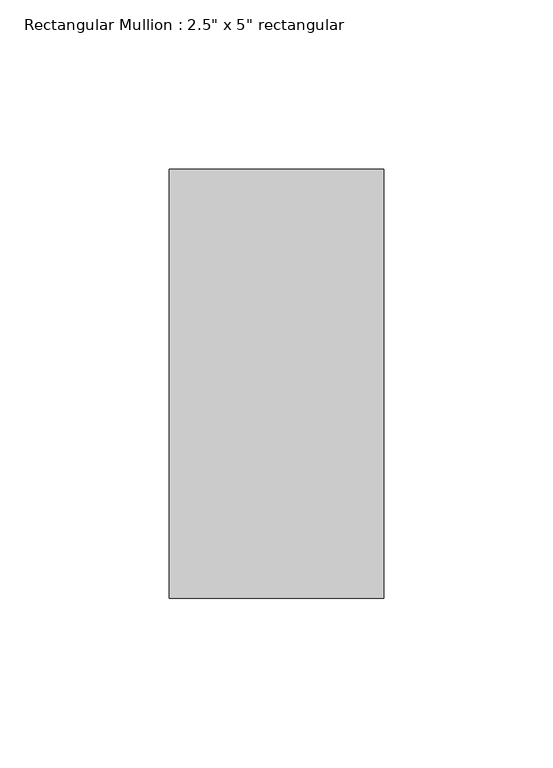
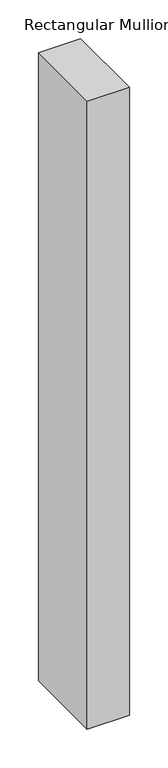
"""IFC4 building model written with IfcOpenShell, lengths in millimetres: member geometry."""

from ifc_helpers import new_model, si_unit, frame, origin, place, context, project, spatial, polyline, outline, extrude, source, transform, mapped, element, save


def member_8f31a534(model_context):
    return source(origin(), model_context, "Body", "SweptSolid", [
        extrude(outline(polyline([(31.75, 63.5), (31.75, -63.5), (-31.75, -63.5), (-31.75, 63.5), (31.75, 63.5)])), frame((0.0, 0.0, -995.2680153), z_axis=(0.0, 0.0, 1.0), x_axis=(1.0, 0.0, 0.0)), (0.0, 0.0, 1.0), 995.2680153),
    ])


if __name__ == "__main__":
    model = new_model("IFC4")
    model_context = context("Model", 3, world=origin())
    ifc_project = project(units=[si_unit("LENGTHUNIT", "METRE", prefix="MILLI")], contexts=[model_context])
    site = spatial("IfcSite", under=ifc_project)
    building = spatial("IfcBuilding", under=site)
    placement = place(None, origin())
    member_shape = member_8f31a534(model_context)
    element("IfcMember", 1, ObjectType="Rectangular Mullion : 2.5\" x 5\" rectangular", at=placement, inside=building, context=model_context, shape_type="MappedRepresentation", body=[
        mapped(member_shape, transform((0.0, 0.0, 0.0), x_axis=(1.0, 0.0, 0.0), y_axis=(0.0, 1.0, 0.0), z_axis=(0.0, 0.0, 1.0))),
    ])
    save(model, "model.ifc")

# Revit data of these elements
# Type "Rectangular Mullion : 2.5\" x 5\" rectangular"
#   built-in parameter 1007304 = 0.416667 (stored number, unit not read)
#   built-in parameter 1007301 = 0.104167 (stored number, unit not read)
#   built-in parameter 1007300 = 0.104167 (stored number, unit not read)
# Element 1 (IfcMember, "Rectangular Mullion : 2.5\" x 5\" rectangular")
#   Materials on its faces: "Aluminum"
# Materials
#   "Aluminum": class "Metal", colour RGB 247 247 247, transparency 0, Description = "Aluminum 6061", Cost = 0
